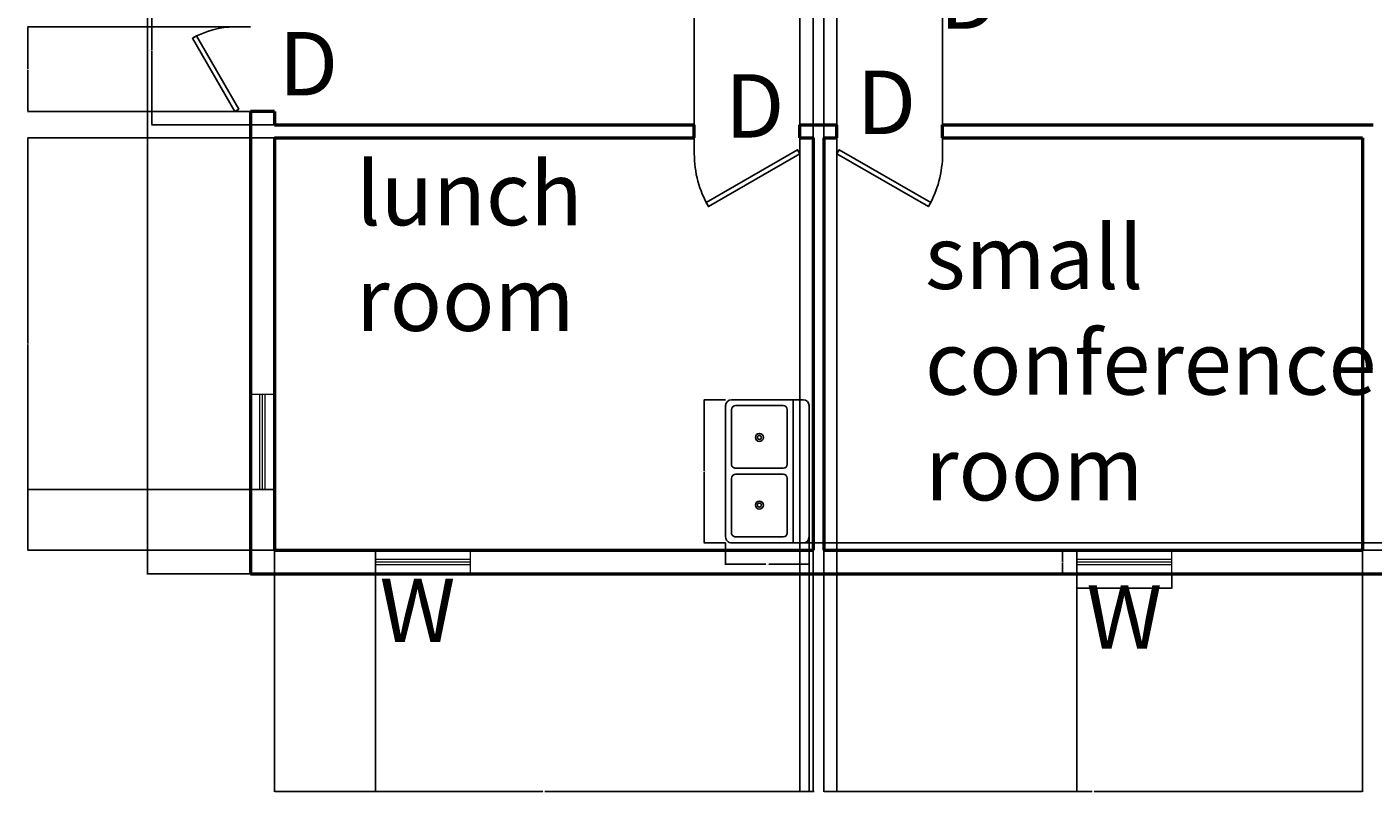
# Model space of a CAD drawing. Units: inches. Extents: x -84 to 931, y 65 to 668.
# Tile 1 of 5: x -84 to 426, y 65 to 355. Entities that reach past the tile are written whole.
import ezdxf

# ---------------------------------------------------------------- set-up
doc = ezdxf.new("R2010")
doc.units = ezdxf.units.IN
doc.header["$MEASUREMENT"] = 0
for name, color, linetype, lineweight in [('A-ANNO-DIMS', 2, 'Continuous', 18), ('A-ANNO-TEXT', 7, 'Continuous', 18), ('A-AREA-IDEN', 7, 'Continuous', 25), ('A-DOOR', 4, 'Continuous', 25), ('A-FLOR-FIXT', 9, 'Continuous', 25), ('A-GLAZ', 4, 'Continuous', 18), ('A-WALL', 7, 'Continuous', 50)]:
    doc.layers.add(name, color=color, linetype=linetype, lineweight=lineweight)
doc.styles.get("Standard").update_dxf_attribs({"font": 'arial.ttf'})
doc.dimstyles.get("Standard").update_dxf_attribs({"dimtxt": 0.18, "dimasz": 0.18, "dimexe": 0.18, "dimexo": 0.0625, "dimgap": 0.09, "dimtad": 0, "dimtih": 1, "dimtoh": 1, "dimdec": 0, "dimzin": 0, "dimdsep": 46, "dimlunit": 3, "dimtxsty": 'Standard', "dimcen": 0.09, "dimadec": 0, "dimazin": 0, "dimtfac": 1, "dimtdec": 0, "dimtofl": 0, "dimtmove": 0, "dimatfit": 3, "dimfxl": 1, "dimtolj": 1, "dimtzin": 0, "dimarcsym": 0})

# ---------------------------------------------------------------- blocks, each defined once
blk = doc.blocks.new('*U9')
for p, q in [((-40, 0), (-40, 6)), ((0, 0), (0, 6))]:
    blk.add_line(p, q)
blk.add_lwpolyline([(0, 0), (-34.64, -20), (-35.52, -18.48), (-0.88, 1.52)], close=True)
blk.add_arc((0, 0), 40, 180, 210)
blk = doc.blocks.new('*U10')
for p, q in [((0, 0), (0, 6)), ((40, 0), (40, 6))]:
    blk.add_line(p, q)
blk.add_lwpolyline([(0, 0), (34.64, -20), (35.52, -18.48), (0.87, 1.52)], close=True)
blk.add_arc((0, 0), 40, 330, 0)
blk = doc.blocks.new('*U11')
for p, q in [((0, 0), (0, -6)), ((32, 0), (32, -6))]:
    blk.add_line(p, q)
blk.add_lwpolyline([(0, 0), (27.71, 16), (28.59, 14.48), (0.87, -1.52)], close=True)
blk.add_arc((0, 0), 32, 0, 30)
blk = doc.blocks.new('Sink-double - 36 in top')
for p, q in [((-18, -4), (18, -4)), ((-0.75, -18.5), (-0.75, -6.5)), ((0.75, -6.5), (0.75, -18.5))]:
    blk.add_line(p, q)
for points in [[(-16.5, 0), (16.5, 0)], [(-18, -19.5), (-18, -1.5)], [(18, -1.5), (18, -19.5)], [(-16.5, -18.5), (-16.5, -6.5)], [(-15.5, -5.5), (-1.75, -5.5)], [(1.75, -5.5), (15.5, -5.5)], [(16.5, -6.5), (16.5, -18.5)], [(-1.75, -19.5), (-15.5, -19.5)], [(15.5, -19.5), (1.75, -19.5)], [(16.5, -21), (-16.5, -21)]]:
    blk.add_lwpolyline(points)
for centre, radius in [((-8.5, -12.5), 1), ((-8.5, -12.5), 0.5), ((8.5, -12.5), 1), ((8.5, -12.5), 0.5)]:
    blk.add_circle(centre, radius)
for centre, radius, start, end in [((-16.5, -1.5), 1.5, 90, 180), ((16.5, -1.5), 1.5, 0, 90), ((-15.5, -6.5), 1, 90, 180), ((-1.75, -6.5), 1, 0, 90), ((1.75, -6.5), 1, 90, 180), ((15.5, -6.5), 1, 0, 90), ((-16.5, -19.5), 1.5, 180, 270), ((-15.5, -18.5), 1, 180, 270), ((-1.75, -18.5), 1, 270, 0), ((1.75, -18.5), 1, 180, 270), ((15.5, -18.5), 1, 270, 0), ((16.5, -19.5), 1.5, 270, 0)]:
    blk.add_arc(centre, radius, start, end)
blk = doc.blocks.new('*D18')
at = {"layer": 'A-ANNO-DIMS', "color": 0, "lineweight": -2, "transparency": 16777216}
for p, q in [((0.47, 603.52), (-38.72, 603.52)), ((-38.54, 603.34), (-38.54, 387.87)), ((-38.54, 147.7), (-38.54, 363.16)), ((0.47, 147.52), (-38.72, 147.52))]:
    blk.add_line(p, q, dxfattribs=at)
at = {"layer": 'A-ANNO-DIMS', "color": 0, "transparency": 16777216}
for points in [[(-38.57, 603.34), (-38.51, 603.34), (-38.54, 603.52)], [(-38.57, 147.7), (-38.51, 147.7), (-38.54, 147.52)]]:
    blk.add_solid(points, dxfattribs=at)
at = {"layer": 'Defpoints', "color": 0, "transparency": 16777216}
for p in [(0.53, 603.52), (-38.54, 147.52), (0.53, 147.52)]:
    blk.add_point(p, dxfattribs=at)
at = {"layer": 'A-ANNO-DIMS', "color": 0, "transparency": 16777216, "insert": (-38.54, 375.52), "char_height": 0.18, "attachment_point": 5}
blk.add_mtext("\\A1;{\\H133.33333x;38'}", dxfattribs=at)
blk = doc.blocks.new('WIN-36IN')
for p, q in [((3.5, 0), (3.5, 36)), ((4.5, 0), (4.5, 36)), ((5.5, 0), (5.5, 36))]:
    blk.add_line(p, q)
blk.add_lwpolyline([(0, 36), (0, 0), (9, 0), (9, 36)], close=True)
blk = doc.blocks.new('*D21')
at = {"layer": 'A-ANNO-DIMS', "color": 0, "lineweight": -2, "transparency": 16777216}
for p, q in [((313.36, 147.45), (313.36, 141.94)), ((349.36, 147.45), (349.36, 141.94)), ((313.54, 142.12), (330.13, 142.12)), ((349.18, 142.12), (332.58, 142.12))]:
    blk.add_line(p, q, dxfattribs=at)
at = {"layer": 'A-ANNO-DIMS', "color": 0, "transparency": 16777216}
for points in [[(313.54, 142.15), (313.54, 142.09), (313.36, 142.12)], [(349.18, 142.15), (349.18, 142.09), (349.36, 142.12)]]:
    blk.add_solid(points, dxfattribs=at)
at = {"layer": 'Defpoints', "color": 0, "transparency": 16777216}
for p in [(313.36, 147.52), (349.36, 147.52), (349.36, 142.12)]:
    blk.add_point(p, dxfattribs=at)
at = {"layer": 'A-ANNO-DIMS', "color": 0, "transparency": 16777216, "insert": (331.36, 142.12), "char_height": 0.18, "attachment_point": 5}
blk.add_mtext('\\A1;WINDOW 3\'-0" TYP.', dxfattribs=at)
blk = doc.blocks.new('*D22')
at = {"layer": 'A-ANNO-DIMS', "color": 0, "lineweight": -2, "transparency": 16777216}
for p, q in [((313.29, 156.52), (307.78, 156.52)), ((307.96, 156.34), (307.96, 152.2)), ((307.96, 147.7), (307.96, 151.83)), ((313.29, 147.52), (307.78, 147.52))]:
    blk.add_line(p, q, dxfattribs=at)
at = {"layer": 'A-ANNO-DIMS', "color": 0, "transparency": 16777216}
for points in [[(307.93, 156.34), (307.99, 156.34), (307.96, 156.52)], [(307.93, 147.7), (307.99, 147.7), (307.96, 147.52)]]:
    blk.add_solid(points, dxfattribs=at)
at = {"layer": 'Defpoints', "color": 0, "transparency": 16777216}
for p in [(313.36, 156.52), (307.96, 147.52), (313.36, 147.52)]:
    blk.add_point(p, dxfattribs=at)
at = {"layer": 'A-ANNO-DIMS', "color": 0, "transparency": 16777216, "insert": (307.96, 152.02), "char_height": 0.18, "attachment_point": 5}
blk.add_mtext('\\A1;0\'-9" TYP.', dxfattribs=at)
blk = doc.blocks.new('*D31')
at = {"layer": 'A-ANNO-DIMS', "color": 0, "lineweight": -2, "transparency": 16777216}
for p, q in [((180.33, 213.42), (172.08, 213.42)), ((172.26, 213.24), (172.26, 186.51)), ((172.26, 159.42), (172.26, 186.15)), ((180.33, 159.24), (172.08, 159.24))]:
    blk.add_line(p, q, dxfattribs=at)
at = {"layer": 'A-ANNO-DIMS', "color": 0, "transparency": 16777216}
for points in [[(172.23, 213.24), (172.29, 213.24), (172.26, 213.42)], [(172.23, 159.42), (172.29, 159.42), (172.26, 159.24)]]:
    blk.add_solid(points, dxfattribs=at)
at = {"layer": 'Defpoints', "color": 0, "transparency": 16777216}
for p in [(180.39, 213.42), (172.26, 159.24), (180.39, 159.24)]:
    blk.add_point(p, dxfattribs=at)
at = {"layer": 'A-ANNO-DIMS', "color": 0, "transparency": 16777216, "insert": (172.26, 186.33), "char_height": 0.18, "attachment_point": 5}
blk.add_mtext('\\A1;DOUBLE SINK 4\'-6"', dxfattribs=at)
blk = doc.blocks.new('*D32')
at = {"layer": 'A-ANNO-DIMS', "color": 0, "lineweight": -2, "transparency": 16777216}
for p, q in [((180.39, 159.18), (180.39, 150.93)), ((211.99, 159.18), (211.99, 150.93)), ((180.57, 151.11), (195.65, 151.11)), ((211.81, 151.11), (196.73, 151.11))]:
    blk.add_line(p, q, dxfattribs=at)
at = {"layer": 'A-ANNO-DIMS', "color": 0, "transparency": 16777216}
for points in [[(180.57, 151.14), (180.57, 151.08), (180.39, 151.11)], [(211.81, 151.14), (211.81, 151.08), (211.99, 151.11)]]:
    blk.add_solid(points, dxfattribs=at)
at = {"layer": 'Defpoints', "color": 0, "transparency": 16777216}
for p in [(180.39, 159.24), (211.99, 159.24), (211.99, 151.11)]:
    blk.add_point(p, dxfattribs=at)
at = {"layer": 'A-ANNO-DIMS', "color": 0, "transparency": 16777216, "insert": (196.19, 151.11), "char_height": 0.18, "attachment_point": 5}
blk.add_mtext('\\A1;2\'-7 1/2"', dxfattribs=at)
blk = doc.blocks.new('*D41')
at = {"layer": 'A-ANNO-DIMS', "color": 0, "lineweight": -2, "transparency": 16777216}
for p, q in [((9.53, 156.45), (9.53, 64.99)), ((213.53, 156.45), (213.53, 64.99)), ((9.71, 65.17), (111.14, 65.17)), ((213.35, 65.17), (111.92, 65.17))]:
    blk.add_line(p, q, dxfattribs=at)
at = {"layer": 'A-ANNO-DIMS', "color": 0, "transparency": 16777216}
for points in [[(9.71, 65.2), (9.71, 65.14), (9.53, 65.17)], [(213.35, 65.2), (213.35, 65.14), (213.53, 65.17)]]:
    blk.add_solid(points, dxfattribs=at)
at = {"layer": 'Defpoints', "color": 0, "transparency": 16777216}
for p in [(9.53, 156.52), (213.53, 156.52), (213.53, 65.17)]:
    blk.add_point(p, dxfattribs=at)
at = {"layer": 'A-ANNO-DIMS', "color": 0, "transparency": 16777216, "insert": (111.53, 65.17), "char_height": 0.18, "attachment_point": 5}
blk.add_mtext('\\A1;17\'-0"', dxfattribs=at)
blk = doc.blocks.new('*D42')
at = {"layer": 'A-ANNO-DIMS', "color": 0, "lineweight": -2, "transparency": 16777216}
for p, q in [((217.53, 156.45), (217.53, 64.99)), ((421.53, 156.45), (421.53, 64.99)), ((217.71, 65.17), (319.14, 65.17)), ((421.35, 65.17), (319.92, 65.17))]:
    blk.add_line(p, q, dxfattribs=at)
at = {"layer": 'A-ANNO-DIMS', "color": 0, "transparency": 16777216}
for points in [[(217.71, 65.2), (217.71, 65.14), (217.53, 65.17)], [(421.35, 65.2), (421.35, 65.14), (421.53, 65.17)]]:
    blk.add_solid(points, dxfattribs=at)
at = {"layer": 'Defpoints', "color": 0, "transparency": 16777216}
for p in [(217.53, 156.52), (421.53, 156.52), (421.53, 65.17)]:
    blk.add_point(p, dxfattribs=at)
at = {"layer": 'A-ANNO-DIMS', "color": 0, "transparency": 16777216, "insert": (319.53, 65.17), "char_height": 0.18, "attachment_point": 5}
blk.add_mtext('\\A1;17\'-0"', dxfattribs=at)
blk = doc.blocks.new('*D47')
at = {"layer": 'A-ANNO-DIMS', "color": 0, "lineweight": -2, "transparency": 16777216}
for p, q in [((9.47, 373.52), (-37, 373.52)), ((-36.82, 373.34), (-36.82, 345.7)), ((-36.82, 317.7), (-36.82, 345.33)), ((9.47, 317.52), (-37, 317.52))]:
    blk.add_line(p, q, dxfattribs=at)
at = {"layer": 'A-ANNO-DIMS', "color": 0, "transparency": 16777216}
for points in [[(-36.85, 373.34), (-36.79, 373.34), (-36.82, 373.52)], [(-36.85, 317.7), (-36.79, 317.7), (-36.82, 317.52)]]:
    blk.add_solid(points, dxfattribs=at)
at = {"layer": 'Defpoints', "color": 0, "transparency": 16777216}
for p in [(-36.82, 373.52), (9.53, 373.52), (9.53, 317.52)]:
    blk.add_point(p, dxfattribs=at)
at = {"layer": 'A-ANNO-DIMS', "color": 0, "transparency": 16777216, "insert": (-36.82, 345.52), "char_height": 0.18, "attachment_point": 5}
blk.add_mtext('\\A1;4\'-8"', dxfattribs=at)
blk = doc.blocks.new('*D48')
at = {"layer": 'A-ANNO-DIMS', "color": 0, "lineweight": -2, "transparency": 16777216}
for p, q in [((9.47, 312.52), (-84, 312.52)), ((-83.82, 312.34), (-83.82, 234.7)), ((-83.82, 156.7), (-83.82, 234.33)), ((9.47, 156.52), (-84, 156.52))]:
    blk.add_line(p, q, dxfattribs=at)
at = {"layer": 'A-ANNO-DIMS', "color": 0, "transparency": 16777216}
for points in [[(-83.85, 312.34), (-83.79, 312.34), (-83.82, 312.52)], [(-83.85, 156.7), (-83.79, 156.7), (-83.82, 156.52)]]:
    blk.add_solid(points, dxfattribs=at)
at = {"layer": 'Defpoints', "color": 0, "transparency": 16777216}
for p in [(9.53, 312.52), (-83.82, 156.52), (9.53, 156.52)]:
    blk.add_point(p, dxfattribs=at)
at = {"layer": 'A-ANNO-DIMS', "color": 0, "transparency": 16777216, "insert": (-83.82, 234.52), "char_height": 0.18, "attachment_point": 5}
blk.add_mtext('\\A1;13\'-0"', dxfattribs=at)
blk = doc.blocks.new('*D52')
at = {"layer": 'A-ANNO-DIMS', "color": 0, "lineweight": -2, "transparency": 16777216}
for p, q in [((0.47, 354.52), (-84, 354.52)), ((-83.82, 354.34), (-83.82, 338.7)), ((-83.82, 322.7), (-83.82, 338.33)), ((0.47, 322.52), (-84, 322.52))]:
    blk.add_line(p, q, dxfattribs=at)
at = {"layer": 'A-ANNO-DIMS', "color": 0, "transparency": 16777216}
for points in [[(-83.85, 354.34), (-83.79, 354.34), (-83.82, 354.52)], [(-83.85, 322.7), (-83.79, 322.7), (-83.82, 322.52)]]:
    blk.add_solid(points, dxfattribs=at)
at = {"layer": 'Defpoints', "color": 0, "transparency": 16777216}
for p in [(-83.82, 354.52), (0.53, 354.52), (0.53, 322.52)]:
    blk.add_point(p, dxfattribs=at)
at = {"layer": 'A-ANNO-DIMS', "color": 0, "transparency": 16777216, "insert": (-83.82, 338.52), "char_height": 0.18, "attachment_point": 5}
blk.add_mtext('\\A1;2\'-8"', dxfattribs=at)
blk = doc.blocks.new('*D56')
at = {"layer": 'A-ANNO-DIMS', "color": 0, "lineweight": -2, "transparency": 16777216}
for p, q in [((9.53, 156.45), (9.53, 64.99)), ((47.8, 156.45), (47.8, 64.99)), ((9.71, 65.17), (28.12, 65.17)), ((47.62, 65.17), (29.2, 65.17))]:
    blk.add_line(p, q, dxfattribs=at)
at = {"layer": 'A-ANNO-DIMS', "color": 0, "transparency": 16777216}
for points in [[(9.71, 65.2), (9.71, 65.14), (9.53, 65.17)], [(47.62, 65.2), (47.62, 65.14), (47.8, 65.17)]]:
    blk.add_solid(points, dxfattribs=at)
at = {"layer": 'Defpoints', "color": 0, "transparency": 16777216}
for p in [(9.53, 156.52), (47.8, 156.52), (47.8, 65.17)]:
    blk.add_point(p, dxfattribs=at)
at = {"layer": 'A-ANNO-DIMS', "color": 0, "transparency": 16777216, "insert": (28.66, 65.17), "char_height": 0.18, "attachment_point": 5}
blk.add_mtext('\\A1;3\'-2 1/2"', dxfattribs=at)
blk = doc.blocks.new('*D57')
at = {"layer": 'A-ANNO-DIMS', "color": 0, "lineweight": -2, "transparency": 16777216}
for p, q in [((217.53, 156.45), (217.53, 64.99)), ((313.36, 156.45), (313.36, 64.99)), ((217.71, 65.17), (265.11, 65.17)), ((313.18, 65.17), (265.77, 65.17))]:
    blk.add_line(p, q, dxfattribs=at)
at = {"layer": 'A-ANNO-DIMS', "color": 0, "transparency": 16777216}
for points in [[(217.71, 65.2), (217.71, 65.14), (217.53, 65.17)], [(313.18, 65.2), (313.18, 65.14), (313.36, 65.17)]]:
    blk.add_solid(points, dxfattribs=at)
at = {"layer": 'Defpoints', "color": 0, "transparency": 16777216}
for p in [(217.53, 156.52), (313.36, 156.52), (313.36, 65.17)]:
    blk.add_point(p, dxfattribs=at)
at = {"layer": 'A-ANNO-DIMS', "color": 0, "transparency": 16777216, "insert": (265.44, 65.17), "char_height": 0.18, "attachment_point": 5}
blk.add_mtext('\\A1;8\'-0"', dxfattribs=at)
blk = doc.blocks.new('*D61')
at = {"layer": 'A-ANNO-DIMS', "color": 0, "lineweight": -2, "transparency": 16777216}
for p, q in [((9.47, 179.37), (-84, 179.37)), ((-83.82, 179.19), (-83.82, 168.12)), ((-83.82, 156.7), (-83.82, 167.76)), ((9.47, 156.52), (-84, 156.52))]:
    blk.add_line(p, q, dxfattribs=at)
at = {"layer": 'A-ANNO-DIMS', "color": 0, "transparency": 16777216}
for points in [[(-83.85, 179.19), (-83.79, 179.19), (-83.82, 179.37)], [(-83.85, 156.7), (-83.79, 156.7), (-83.82, 156.52)]]:
    blk.add_solid(points, dxfattribs=at)
at = {"layer": 'Defpoints', "color": 0, "transparency": 16777216}
for p in [(-83.82, 179.37), (9.53, 179.37), (9.53, 156.52)]:
    blk.add_point(p, dxfattribs=at)
at = {"layer": 'A-ANNO-DIMS', "color": 0, "transparency": 16777216, "insert": (-83.82, 167.94), "char_height": 0.18, "attachment_point": 5}
blk.add_mtext('\\A1;1\'-11"', dxfattribs=at)
blk = doc.blocks.new('*D69')
at = {"layer": 'A-ANNO-DIMS', "color": 0, "lineweight": -2, "transparency": 16777216}
for p, q in [((168.52, 312.58), (168.52, 650.05)), ((168.7, 649.87), (188.2, 649.87)), ((208.35, 649.87), (188.86, 649.87)), ((208.53, 312.58), (208.53, 650.05))]:
    blk.add_line(p, q, dxfattribs=at)
at = {"layer": 'A-ANNO-DIMS', "color": 0, "transparency": 16777216}
for points in [[(168.7, 649.9), (168.7, 649.84), (168.52, 649.87)], [(208.35, 649.9), (208.35, 649.84), (208.53, 649.87)]]:
    blk.add_solid(points, dxfattribs=at)
at = {"layer": 'Defpoints', "color": 0, "transparency": 16777216}
for p in [(208.53, 649.87), (168.52, 312.52), (208.53, 312.52)]:
    blk.add_point(p, dxfattribs=at)
at = {"layer": 'A-ANNO-DIMS', "color": 0, "transparency": 16777216, "insert": (188.53, 649.87), "char_height": 0.18, "attachment_point": 5}
blk.add_mtext('\\A1;3\'-4"', dxfattribs=at)
blk = doc.blocks.new('*D70')
at = {"layer": 'A-ANNO-DIMS', "color": 0, "lineweight": -2, "transparency": 16777216}
for p, q in [((222.53, 312.58), (222.53, 650.05)), ((222.71, 649.87), (242.2, 649.87)), ((262.35, 649.87), (242.86, 649.87)), ((262.53, 312.58), (262.53, 650.05))]:
    blk.add_line(p, q, dxfattribs=at)
at = {"layer": 'A-ANNO-DIMS', "color": 0, "transparency": 16777216}
for points in [[(222.71, 649.9), (222.71, 649.84), (222.53, 649.87)], [(262.35, 649.9), (262.35, 649.84), (262.53, 649.87)]]:
    blk.add_solid(points, dxfattribs=at)
at = {"layer": 'Defpoints', "color": 0, "transparency": 16777216}
for p in [(262.53, 649.87), (222.53, 312.52), (262.53, 312.52)]:
    blk.add_point(p, dxfattribs=at)
at = {"layer": 'A-ANNO-DIMS', "color": 0, "transparency": 16777216, "insert": (242.53, 649.87), "char_height": 0.18, "attachment_point": 5}
blk.add_mtext('\\A1;3\'-4"', dxfattribs=at)
blk = doc.blocks.new('*D71')
at = {"layer": 'A-ANNO-DIMS', "color": 0, "lineweight": -2, "transparency": 16777216}
for p, q in [((208.53, 312.45), (208.53, 64.99)), ((213.53, 312.45), (213.53, 64.99)), ((208.71, 65.17), (210.7, 65.17)), ((213.35, 65.17), (211.36, 65.17))]:
    blk.add_line(p, q, dxfattribs=at)
at = {"layer": 'A-ANNO-DIMS', "color": 0, "transparency": 16777216}
for points in [[(208.71, 65.2), (208.71, 65.14), (208.53, 65.17)], [(213.35, 65.2), (213.35, 65.14), (213.53, 65.17)]]:
    blk.add_solid(points, dxfattribs=at)
at = {"layer": 'Defpoints', "color": 0, "transparency": 16777216}
for p in [(208.53, 312.52), (213.53, 312.52), (213.53, 65.17)]:
    blk.add_point(p, dxfattribs=at)
at = {"layer": 'A-ANNO-DIMS', "color": 0, "transparency": 16777216, "insert": (211.03, 65.17), "char_height": 0.18, "attachment_point": 5}
blk.add_mtext('\\A1;0\'-5"', dxfattribs=at)
blk = doc.blocks.new('*D72')
at = {"layer": 'A-ANNO-DIMS', "color": 0, "lineweight": -2, "transparency": 16777216}
for p, q in [((217.53, 312.45), (217.53, 64.99)), ((222.53, 312.45), (222.53, 64.99)), ((217.71, 65.17), (219.7, 65.17)), ((222.35, 65.17), (220.36, 65.17))]:
    blk.add_line(p, q, dxfattribs=at)
at = {"layer": 'A-ANNO-DIMS', "color": 0, "transparency": 16777216}
for points in [[(217.71, 65.2), (217.71, 65.14), (217.53, 65.17)], [(222.35, 65.2), (222.35, 65.14), (222.53, 65.17)]]:
    blk.add_solid(points, dxfattribs=at)
at = {"layer": 'Defpoints', "color": 0, "transparency": 16777216}
for p in [(217.53, 312.52), (222.53, 312.52), (222.53, 65.17)]:
    blk.add_point(p, dxfattribs=at)
at = {"layer": 'A-ANNO-DIMS', "color": 0, "transparency": 16777216, "insert": (220.03, 65.17), "char_height": 0.18, "attachment_point": 5}
blk.add_mtext('\\A1;0\'-5"', dxfattribs=at)
blk = doc.blocks.new('*D73')
at = {"layer": 'A-ANNO-DIMS', "color": 0, "lineweight": -2, "transparency": 16777216}
for p, q in [((213.53, 156.58), (213.53, 650.05)), ((213.71, 649.87), (215.2, 649.87)), ((217.35, 649.87), (215.86, 649.87)), ((217.53, 156.58), (217.53, 650.05))]:
    blk.add_line(p, q, dxfattribs=at)
at = {"layer": 'A-ANNO-DIMS', "color": 0, "transparency": 16777216}
for points in [[(213.71, 649.9), (213.71, 649.84), (213.53, 649.87)], [(217.35, 649.9), (217.35, 649.84), (217.53, 649.87)]]:
    blk.add_solid(points, dxfattribs=at)
at = {"layer": 'Defpoints', "color": 0, "transparency": 16777216}
for p in [(217.53, 649.87), (213.53, 156.52), (217.53, 156.52)]:
    blk.add_point(p, dxfattribs=at)
at = {"layer": 'A-ANNO-DIMS', "color": 0, "transparency": 16777216, "insert": (215.53, 649.87), "char_height": 0.18, "attachment_point": 5}
blk.add_mtext('\\A1;0\'-4"', dxfattribs=at)
blk = doc.blocks.new('*D77')
at = {"layer": 'A-ANNO-DIMS', "color": 0, "lineweight": -2, "transparency": 16777216}
for p, q in [((211.99, 161.43), (211.99, 64.99)), ((213.53, 156.45), (213.53, 64.99)), ((211.81, 65.17), (211.63, 65.17)), ((213.71, 65.17), (213.89, 65.17))]:
    blk.add_line(p, q, dxfattribs=at)
at = {"layer": 'A-ANNO-DIMS', "color": 0, "transparency": 16777216}
for points in [[(211.81, 65.2), (211.81, 65.14), (211.99, 65.17)], [(213.71, 65.2), (213.71, 65.14), (213.53, 65.17)]]:
    blk.add_solid(points, dxfattribs=at)
at = {"layer": 'Defpoints', "color": 0, "transparency": 16777216}
for p in [(211.99, 161.5), (213.53, 156.52), (213.53, 65.17)]:
    blk.add_point(p, dxfattribs=at)
at = {"layer": 'A-ANNO-DIMS', "color": 0, "transparency": 16777216, "insert": (212.76, 65.17), "char_height": 0.18, "attachment_point": 5}
blk.add_mtext('\\A1;0\'-1 1/2"', dxfattribs=at)
blk = doc.blocks.new('*D78')
at = {"layer": 'A-ANNO-DIMS', "color": 0, "lineweight": -2, "transparency": 16777216}
for p, q in [((182.71, 159.24), (931.06, 159.24)), ((930.88, 159.06), (930.88, 158.06)), ((217.59, 156.52), (931.06, 156.52)), ((930.88, 156.7), (930.88, 157.69))]:
    blk.add_line(p, q, dxfattribs=at)
at = {"layer": 'A-ANNO-DIMS', "color": 0, "transparency": 16777216}
for points in [[(930.85, 159.06), (930.91, 159.06), (930.88, 159.24)], [(930.85, 156.7), (930.91, 156.7), (930.88, 156.52)]]:
    blk.add_solid(points, dxfattribs=at)
at = {"layer": 'Defpoints', "color": 0, "transparency": 16777216}
for p in [(182.65, 159.24), (217.53, 156.52), (930.88, 156.52)]:
    blk.add_point(p, dxfattribs=at)
at = {"layer": 'A-ANNO-DIMS', "color": 0, "transparency": 16777216, "insert": (930.88, 157.88), "char_height": 0.18, "attachment_point": 5}
blk.add_mtext('\\A1;0\'-2 1/2"', dxfattribs=at)

msp = doc.modelspace()

# ---------------------------------------------------------------- linework, layer by layer
at = {"layer": 'A-WALL'}
for p, q in [((9.53, 322.52), (0.53, 322.52)), ((0.53, 322.52), (0.53, 317.52)), ((9.53, 322.52), (9.53, 317.52)), ((0.53, 317.52), (0.53, 147.52)), ((9.53, 317.52), (168.52, 317.52)), ((168.52, 312.52), (168.52, 317.52)), ((208.53, 312.52), (208.53, 317.52)), ((208.53, 317.52), (222.53, 317.52)), ((222.53, 312.52), (222.53, 317.52)), ((262.53, 312.52), (262.53, 317.52)), ((262.53, 317.52), (425.53, 317.52)), ((9.53, 312.52), (168.52, 312.52)), ((9.53, 312.52), (9.53, 156.52)), ((208.52, 312.52), (213.53, 312.52)), ((213.53, 312.52), (213.53, 156.52)), ((217.53, 312.52), (217.53, 156.52)), ((217.53, 312.52), (222.53, 312.52)), ((262.53, 312.52), (421.53, 312.52)), ((421.53, 312.52), (421.53, 156.52)), ((9.53, 156.52), (213.53, 156.52)), ((217.53, 156.52), (421.53, 156.52)), ((0.53, 147.52), (431.53, 147.52))]:
    msp.add_line(p, q, dxfattribs=at)

# ---------------------------------------------------------------- block references
at = {"layer": 'A-DOOR', "rotation": 90}
msp.add_blockref('*U11', (-5.47, 322.52), dxfattribs=at)
at = {"layer": 'A-DOOR'}
for name, p in [('*U9', (208.52, 306.52)), ('*U10', (222.53, 306.52))]:
    msp.add_blockref(name, p, dxfattribs=at)
at = {"layer": 'A-FLOR-FIXT', "xscale": 1.505023096701488, "yscale": 1.505023096701488, "zscale": 1.505023096701488, "rotation": 270}
msp.add_blockref('Sink-double - 36 in top', (211.99, 186.33), dxfattribs=at)
at = {"layer": 'A-GLAZ'}
msp.add_blockref('WIN-36IN', (0.53, 179.37), dxfattribs=at)
at = {"layer": 'A-GLAZ', "rotation": 270.0000000000001}
for p in [(47.8, 156.52), (313.36, 156.52)]:
    msp.add_blockref('WIN-36IN', p, dxfattribs=at)

# ---------------------------------------------------------------- texts
at = {"layer": 'A-ANNO-TEXT', "char_height": 24, "attachment_point": 1}
for s, width, insert in [('D', 21.9508, (261.26, 377.82)), ('D', 21.9508, (11.16, 352.58)), ('D', 21.9508, (180.11, 336.63)), ('D', 21.9508, (230, 337.96)), ('W', 20.4711, (49.37, 145.66)), ('W', 20.4711, (316.96, 143.12))]:
    msp.add_mtext_dynamic_manual_height_columns(s, width=width, gutter_width=1, heights=[0], dxfattribs=dict(at, insert=insert))
at = {"layer": 'A-AREA-IDEN', "char_height": 24, "attachment_point": 1}
for s, insert in [('lunch room', (40.48, 303.45)), ('small conference room', (255.87, 279.33))]:
    msp.add_mtext_dynamic_manual_height_columns(s, width=131.8349, gutter_width=1, heights=[0], dxfattribs=dict(at, insert=insert))

# ---------------------------------------------------------------- dimensions: what is measured, and where the dimension line sits
at = {"layer": 'A-ANNO-DIMS'}
for base, p1, p2, picture, middle in [((208.53, 649.87), (168.52, 312.52), (208.53, 312.52), '*D69', (188.53, 649.87)), ((217.53, 649.87), (213.53, 156.52), (217.53, 156.52), '*D73', (215.53, 649.87)), ((262.53, 649.87), (222.53, 312.52), (262.53, 312.52), '*D70', (242.53, 649.87)), ((213.53, 65.17), (208.53, 312.52), (213.53, 312.52), '*D71', (211.03, 65.17)), ((222.53, 65.17), (217.53, 312.52), (222.53, 312.52), '*D72', (220.03, 65.17)), ((211.99, 151.11), (180.39, 159.24), (211.99, 159.24), '*D32', (196.19, 151.11)), ((213.53, 65.17), (211.99, 161.5), (213.53, 156.52), '*D77', (212.76, 65.17)), ((213.53, 65.17), (9.53, 156.52), (213.53, 156.52), '*D41', (111.53, 65.17)), ((47.8, 65.17), (9.53, 156.52), (47.8, 156.52), '*D56', (28.66, 65.17)), ((421.53, 65.17), (217.53, 156.52), (421.53, 156.52), '*D42', (319.53, 65.17)), ((313.36, 65.17), (217.53, 156.52), (313.36, 156.52), '*D57', (265.44, 65.17))]:
    dim = msp.add_linear_dim(base=base, p1=p1, p2=p2, dimstyle='Standard', override={"dimdec": 1, "dimlfac": 1, "dimrnd": 0, "dimzin": 1, "dimdsep": 46, "dimlunit": 4, "dimfrac": 2}, dxfattribs=at)
    dim.commit()
    dim.dimension.update_dxf_attribs({"geometry": picture, "text_midpoint": middle})
for base, p1, p2, angle, text, override, picture, middle in [((-38.54, 147.52), (0.53, 603.52), (0.53, 147.52), 90, '{\\H133.33333x;<>}', {"dimclrd": 0, "dimclre": 0, "dimclrt": 0}, '*D18', (-38.54, 375.52)), ((172.26, 159.24), (180.39, 213.42), (180.39, 159.24), 270, 'DOUBLE SINK <>', {"dimdec": 1, "dimlfac": 1, "dimrnd": 0, "dimzin": 1, "dimdsep": 46, "dimlunit": 4, "dimfrac": 2}, '*D31', (172.26, 186.33)), ((307.96, 147.52), (313.36, 156.52), (313.36, 147.52), 270, '<> TYP.', {"dimdec": 1, "dimlfac": 1, "dimrnd": 0, "dimzin": 1, "dimdsep": 46, "dimlunit": 4, "dimfrac": 2}, '*D22', (307.96, 152.02)), ((349.36, 142.12), (313.36, 147.52), (349.36, 147.52), 0, 'WINDOW <> TYP.', {"dimdec": 1, "dimlfac": 1, "dimrnd": 0, "dimzin": 1, "dimdsep": 46, "dimlunit": 4, "dimfrac": 2}, '*D21', (331.36, 142.12))]:
    dim = msp.add_linear_dim(base=base, p1=p1, p2=p2, angle=angle, text=text, dimstyle='Standard', override=override, dxfattribs=at)
    dim.commit()
    dim.dimension.update_dxf_attribs({"geometry": picture, "text_midpoint": middle})
for base, p1, p2, picture, middle in [((-36.82, 373.52), (9.53, 317.52), (9.53, 373.52), '*D47', (-36.82, 345.52)), ((-83.82, 354.52), (0.53, 322.52), (0.53, 354.52), '*D52', (-83.82, 338.52)), ((-83.82, 156.52), (9.53, 312.52), (9.53, 156.52), '*D48', (-83.82, 234.52)), ((-83.8196, 179.366), (9.5304, 156.5157), (9.5304, 179.366), '*D61', (-83.8196, 167.9409)), ((930.88, 156.52), (182.65, 159.24), (217.53, 156.52), '*D78', (930.88, 157.88))]:
    dim = msp.add_linear_dim(base=base, p1=p1, p2=p2, angle=90, dimstyle='Standard', override={"dimdec": 1, "dimlfac": 1, "dimrnd": 0, "dimzin": 1, "dimdsep": 46, "dimlunit": 4, "dimfrac": 2}, dxfattribs=at)
    dim.commit()
    dim.dimension.update_dxf_attribs({"geometry": picture, "text_midpoint": middle})

doc.saveas('drawing.dxf')
